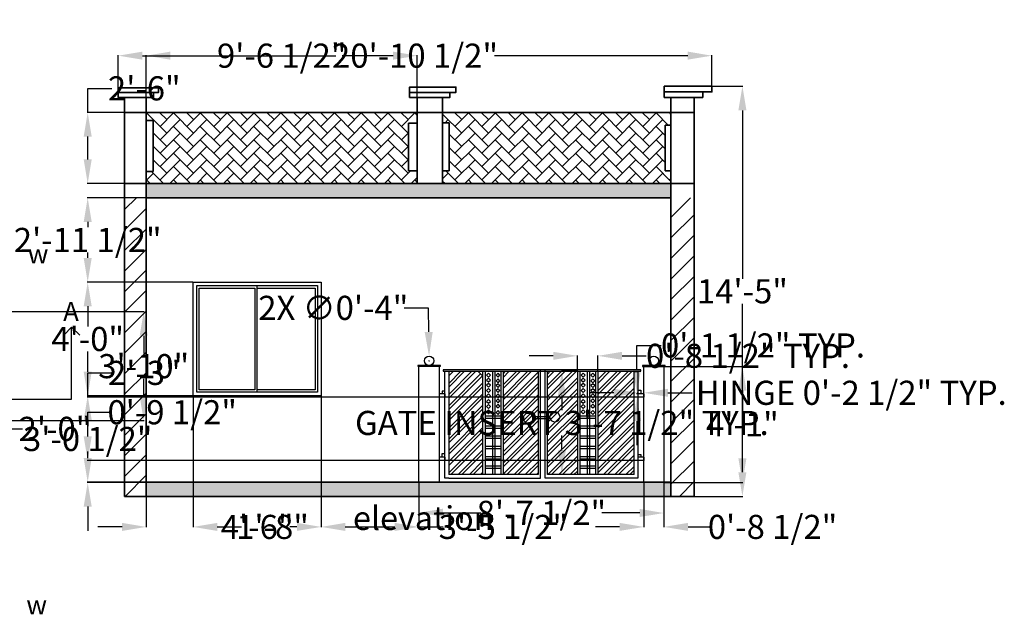
# Model space of a CAD drawing. Units: inches. Extents: x 4451 to 5261, y 886 to 1442.
# Tile 4 of 4: x 4807 to 5223, y 1174 to 1424. Entities that reach past the tile are written whole.
import ezdxf

# ---------------------------------------------------------------- set-up
doc = ezdxf.new("R2010")
doc.units = ezdxf.units.IN
doc.header["$MEASUREMENT"] = 0
for name, color, linetype, lineweight in [('A-ANNO-DIMS', 2, 'Continuous', 18), ('A-ANNO-SYMB', 3, 'Continuous', 25), ('A-ANNO-TEXT', 7, 'Continuous', 25), ('A-ELEV', 7, 'Continuous', 35), ('A-ELEV-GATE', 4, 'Continuous', 25), ('A-GLAZ', 4, 'Continuous', 25)]:
    doc.layers.add(name, color=color, linetype=linetype, lineweight=lineweight)
doc.layers.add('A-ELEV-GATE-PATT', color=30, linetype='Continuous', lineweight=13, true_color=0xf8991e)
doc.layers.add('A-ELEV-PATT', color=240, linetype='Continuous', lineweight=13, true_color=0xed1f24)
doc.styles.get("Standard").update_dxf_attribs({"font": 'arial.ttf'})
doc.dimstyles.get("Standard").update_dxf_attribs({"dimtxt": 10.18, "dimasz": 10.18, "dimexe": 0.18, "dimexo": 0.0625, "dimgap": 0.09, "dimtad": 0, "dimtih": 1, "dimtoh": 1, "dimdec": 0, "dimzin": 0, "dimdsep": 46, "dimlunit": 3, "dimtxsty": 'Standard', "dimcen": 0.09, "dimadec": 0, "dimazin": 0, "dimtfac": 1, "dimtdec": 0, "dimtofl": 0, "dimtmove": 0, "dimatfit": 3, "dimfxl": 1, "dimtolj": 1, "dimtzin": 0, "dimarcsym": 0})
pattern_1 = [(50, (284.271, 536.571), (7.172602, -0.627521), [0.75, -8.25]), (355, (284.271, 536.571), (-1.387513, 7.521921), [0.6, -6.6]), (100.45144, (284.869, 536.519), (5.785088, 6.8944), [0.637402, -7.011421]), (46.1842, (284.271, 538.571), (10.672413, -1.655193), [1.125, -12.375]), (96.63564, (285.16, 538.433), (9.34662, 9.741186), [0.956103, -10.517138]), (351.18416, (284.271, 538.571), (9.34662, 9.741186), [0.9, -9.9]), (21, (285.271, 538.071), (5.9690705, -4.026189), [0.75, -8.25]), (326, (285.271, 538.071), (2.433153, 7.2515), [0.6, -6.6]), (71.45144, (285.7684, 537.7355), (8.402224, 3.225312), [0.637402, -7.011421]), (37.5, (284.271, 536.571), (0.1215986, 3.3289385), [0, -6.52, 0, -6.7, 0, -6.625]), (7.5, (284.271, 536.571), (2.6306954, 3.944117), [0, -3.82, 0, -6.37, 0, -2.525]), (327.5, (282.041, 536.571), (5.3382244, -0.2255487), [0, -2.5, 0, -7.8, 0, -10.35]), (317.5, (281.041, 536.571), (5.8318617, 1.00105), [0, -3.25, 0, -5.18, 0, -7.35])]
pattern_2 = [(45, (284.271, 536.571), (-2.3599689, 2.3599689), []), (45, (285.8443, 536.571), (-2.3599689, 2.3599689), [])]

# ---------------------------------------------------------------- blocks, each defined once
blk = doc.blocks.new('*U9')
for p, q in [((1.5, 1.5), (1.5, 46.5)), ((1.5, 46.5), (27, 46.5)), ((27, 1.5), (27, 46.5)), ((27, 46.5), (52.5, 46.5)), ((52.5, 46.5), (52.5, 1.5)), ((27, 1.5), (1.5, 1.5)), ((52.5, 1.5), (27, 1.5))]:
    blk.add_line(p, q)
blk.add_lwpolyline([(0, 0), (0, 48), (54, 48), (54, 0)], close=True)
for points in [[(26, 45.5), (26, 2.5), (2.5, 2.5), (2.5, 45.5), (26, 45.5)], [(27, 45.5), (51.5, 45.5), (51.5, 2.5), (27, 2.5)]]:
    blk.add_lwpolyline(points)
blk = doc.blocks.new('GATE-ORNAMENTAL-INSERT')
for p, q in [((0, 43.58), (0, 0)), ((1, 43.58), (1, 0)), ((4.1, 43.58), (4.1, 0)), ((5.1, 43.58), (5.1, 0)), ((7.67, 43.58), (7.67, 0)), ((8.67, 43.58), (8.67, 0)), ((1, 24.75), (7.67, 24.75)), ((1, 23.75), (7.67, 23.75)), ((1, 20.57), (7.67, 20.57)), ((1, 19.57), (7.67, 19.57)), ((1, 16.4), (7.67, 16.4)), ((1, 15.4), (7.67, 15.4)), ((1, 12.02), (7.67, 12.02)), ((1, 11.02), (7.67, 11.02)), ((1, 7.67), (7.67, 7.67)), ((1, 6.67), (7.67, 6.67)), ((1, 3.65), (7.67, 3.65)), ((1, 2.65), (7.67, 2.65))]:
    blk.add_line(p, q)
for points in [[(2.44, 41.12), (3.27, 41.95), (2.44, 42.78), (1.61, 41.95)], [(6.48, 41.12), (7.31, 41.95), (6.48, 42.78), (5.65, 41.95)], [(2.44, 39.08), (3.27, 39.9), (2.44, 40.73), (1.61, 39.9)], [(2.44, 36.83), (3.27, 37.66), (2.44, 38.49), (1.61, 37.66)], [(6.48, 38.71), (7.31, 39.54), (6.48, 40.37), (5.65, 39.54)], [(6.48, 36.69), (7.31, 37.52), (6.48, 38.35), (5.65, 37.52)], [(2.44, 34.62), (3.27, 35.45), (2.44, 36.28), (1.61, 35.45)], [(2.44, 32.44), (3.27, 33.26), (2.44, 34.09), (1.61, 33.26)], [(6.48, 34.59), (7.31, 35.42), (6.48, 36.25), (5.65, 35.42)], [(6.48, 32.44), (7.31, 33.27), (6.48, 34.1), (5.65, 33.27)], [(2.44, 30.07), (3.27, 30.9), (2.44, 31.73), (1.61, 30.9)], [(2.44, 27.92), (3.27, 28.74), (2.44, 29.57), (1.61, 28.74)], [(6.48, 30.33), (7.31, 31.16), (6.48, 31.99), (5.65, 31.16)], [(6.48, 28.1), (7.31, 28.93), (6.48, 29.76), (5.65, 28.93)], [(2.44, 25.62), (3.27, 26.45), (2.44, 27.28), (1.61, 26.45)], [(6.48, 25.4), (7.31, 26.23), (6.48, 27.06), (5.65, 26.23)]]:
    blk.add_lwpolyline(points, close=True)
blk = doc.blocks.new('GATE-HINGE-ELEV')
for p, q in [((2.48, 1.41), (0, 1.41)), ((2.48, 1.41), (2.48, 0)), ((2.48, 0), (0, 0))]:
    blk.add_line(p, q)
blk = doc.blocks.new('*D31')
at = {"layer": 'A-ANNO-DIMS', "color": 0, "lineweight": -2, "transparency": 16777216}
for p, q in [((5057.78, 1267), (5047.6, 1267)), ((5067.96, 1266.69), (5067.96, 1267.18)), ((5070.44, 1266.69), (5070.44, 1267.18)), ((5080.62, 1267), (5090.8, 1267))]:
    blk.add_line(p, q, dxfattribs=at)
at = {"layer": 'A-ANNO-DIMS', "color": 0, "transparency": 16777216}
for points in [[(5057.78, 1268.7), (5057.78, 1265.31), (5067.96, 1267)], [(5080.62, 1268.7), (5080.62, 1265.31), (5070.44, 1267)]]:
    blk.add_solid(points, dxfattribs=at)
at = {"layer": 'Defpoints', "color": 0, "transparency": 16777216}
for p in [(5067.96, 1266.63), (5070.44, 1267), (5070.44, 1266.63)]:
    blk.add_point(p, dxfattribs=at)
at = {"layer": 'A-ANNO-DIMS', "color": 0, "transparency": 16777216, "insert": (5158, 1267), "char_height": 10.18, "attachment_point": 5}
blk.add_mtext('\\A1;HINGE 0\'-2 1/2" TYP.', dxfattribs=at)
blk = doc.blocks.new('*D32')
at = {"layer": 'A-ANNO-DIMS', "color": 0, "lineweight": -2, "transparency": 16777216}
for p, q in [((5067.58, 1276.81), (5067.58, 1286.99)), ((5067.58, 1286.99), (5077.76, 1286.99)), ((5067.89, 1266.63), (5067.4, 1266.63)), ((5067.89, 1265.22), (5067.4, 1265.22)), ((5067.58, 1255.04), (5067.58, 1244.86))]:
    blk.add_line(p, q, dxfattribs=at)
at = {"layer": 'A-ANNO-DIMS', "color": 0, "transparency": 16777216}
for points in [[(5065.89, 1276.81), (5069.28, 1276.81), (5067.58, 1266.63)], [(5065.89, 1255.04), (5069.28, 1255.04), (5067.58, 1265.22)]]:
    blk.add_solid(points, dxfattribs=at)
at = {"layer": 'Defpoints', "color": 0, "transparency": 16777216}
for p in [(5067.58, 1266.63), (5067.96, 1266.63), (5067.96, 1265.22)]:
    blk.add_point(p, dxfattribs=at)
at = {"layer": 'A-ANNO-DIMS', "color": 0, "transparency": 16777216, "insert": (5120.74, 1286.99), "char_height": 10.18, "attachment_point": 5}
blk.add_mtext('\\A1;0\'-1 1/2" TYP.', dxfattribs=at)
blk = doc.blocks.new('*D33')
at = {"layer": 'A-ANNO-DIMS', "color": 0, "lineweight": -2, "transparency": 16777216}
for p, q in [((5042.35, 1276.06), (5035.7, 1276.06)), ((5035.88, 1265.88), (5035.88, 1259.63)), ((5035.88, 1242.67), (5035.88, 1248.92)), ((5042.35, 1232.49), (5035.7, 1232.49))]:
    blk.add_line(p, q, dxfattribs=at)
at = {"layer": 'A-ANNO-DIMS', "color": 0, "transparency": 16777216}
for points in [[(5034.18, 1265.88), (5037.57, 1265.88), (5035.88, 1276.06)], [(5034.18, 1242.67), (5037.57, 1242.67), (5035.88, 1232.49)]]:
    blk.add_solid(points, dxfattribs=at)
at = {"layer": 'Defpoints', "color": 0, "transparency": 16777216}
for p in [(5035.88, 1276.06), (5042.41, 1276.06), (5042.41, 1232.49)]:
    blk.add_point(p, dxfattribs=at)
at = {"layer": 'A-ANNO-DIMS', "color": 0, "transparency": 16777216, "insert": (5035.88, 1254.28), "char_height": 10.18, "attachment_point": 5}
blk.add_mtext('\\A1;GATE INSERT 3\'-7 1/2" TYP.', dxfattribs=at)
blk = doc.blocks.new('*D34')
at = {"layer": 'A-ANNO-DIMS', "color": 0, "lineweight": -2, "transparency": 16777216}
for p, q in [((5032.23, 1282.6), (5022.05, 1282.6)), ((5042.41, 1276.13), (5042.41, 1282.78)), ((5051.09, 1276.13), (5051.09, 1282.78)), ((5061.27, 1282.6), (5071.45, 1282.6))]:
    blk.add_line(p, q, dxfattribs=at)
at = {"layer": 'A-ANNO-DIMS', "color": 0, "transparency": 16777216}
for points in [[(5032.23, 1284.3), (5032.23, 1280.9), (5042.41, 1282.6)], [(5061.27, 1284.3), (5061.27, 1280.9), (5051.09, 1282.6)]]:
    blk.add_solid(points, dxfattribs=at)
at = {"layer": 'Defpoints', "color": 0, "transparency": 16777216}
for p in [(5051.09, 1282.6), (5042.41, 1276.06), (5051.09, 1276.06)]:
    blk.add_point(p, dxfattribs=at)
at = {"layer": 'A-ANNO-DIMS', "color": 0, "transparency": 16777216, "insert": (5114.42, 1282.6), "char_height": 10.18, "attachment_point": 5}
blk.add_mtext('\\A1;0\'-8 1/2" TYP.', dxfattribs=at)
blk = doc.blocks.new('*D46')
at = {"layer": 'A-ANNO-DIMS', "color": 0, "lineweight": -2, "transparency": 16777216}
for p, q in [((4798.16, 1301.25), (4859.61, 1301.25)), ((4859.43, 1291.07), (4859.43, 1283.54)), ((4859.43, 1265.43), (4859.43, 1272.96)), ((4798.16, 1255.25), (4859.61, 1255.25))]:
    blk.add_line(p, q, dxfattribs=at)
at = {"layer": 'A-ANNO-DIMS', "color": 0, "transparency": 16777216}
for points in [[(4857.74, 1291.07), (4861.13, 1291.07), (4859.43, 1301.25)], [(4857.74, 1265.43), (4861.13, 1265.43), (4859.43, 1255.25)]]:
    blk.add_solid(points, dxfattribs=at)
at = {"layer": 'Defpoints', "color": 0, "transparency": 16777216}
for p in [(4798.09, 1301.25), (4859.43, 1301.25), (4798.09, 1255.25)]:
    blk.add_point(p, dxfattribs=at)
at = {"layer": 'A-ANNO-DIMS', "color": 0, "transparency": 16777216, "insert": (4859.43, 1278.25), "char_height": 10.18, "attachment_point": 5}
blk.add_mtext('\\A1;3\'-10"', dxfattribs=at)
blk = doc.blocks.new('*D54')
at = {"layer": 'A-ANNO-DIMS', "color": 0, "lineweight": -2, "transparency": 16777216}
for p, q in [((4774.09, 1224.89), (4774.09, 1251.96)), ((4784.27, 1251.78), (4787.91, 1251.78)), ((4798.09, 1224.89), (4798.09, 1251.96)), ((4798.09, 1251.78), (4808.27, 1251.78))]:
    blk.add_line(p, q, dxfattribs=at)
at = {"layer": 'A-ANNO-DIMS', "color": 0, "transparency": 16777216}
for points in [[(4784.27, 1253.48), (4784.27, 1250.08), (4774.09, 1251.78)], [(4787.91, 1253.48), (4787.91, 1250.08), (4798.09, 1251.78)]]:
    blk.add_solid(points, dxfattribs=at)
at = {"layer": 'Defpoints', "color": 0, "transparency": 16777216}
for p in [(4798.09, 1251.78), (4774.09, 1224.83), (4798.09, 1224.83)]:
    blk.add_point(p, dxfattribs=at)
at = {"layer": 'A-ANNO-DIMS', "color": 0, "transparency": 16777216, "insert": (4821.98, 1251.78), "char_height": 10.18, "attachment_point": 5}
blk.add_mtext('\\A1;2\'-0"', dxfattribs=at)
blk = doc.blocks.new('*D57')
at = {"layer": 'A-ANNO-DIMS', "color": 0, "lineweight": -2, "transparency": 16777216}
for p, q in [((4848.69, 1395.83), (4848.69, 1409.46)), ((4858.87, 1409.28), (4940.45, 1409.28)), ((5088.98, 1409.28), (5007.4, 1409.28)), ((5099.16, 1396.45), (5099.16, 1409.46))]:
    blk.add_line(p, q, dxfattribs=at)
at = {"layer": 'A-ANNO-DIMS', "color": 0, "transparency": 16777216}
for points in [[(4858.87, 1410.98), (4858.87, 1407.59), (4848.69, 1409.28)], [(5088.98, 1410.98), (5088.98, 1407.59), (5099.16, 1409.28)]]:
    blk.add_solid(points, dxfattribs=at)
at = {"layer": 'Defpoints', "color": 0, "transparency": 16777216}
for p in [(5099.16, 1409.28), (5099.16, 1396.38), (4848.69, 1395.77)]:
    blk.add_point(p, dxfattribs=at)
at = {"layer": 'A-ANNO-DIMS', "color": 0, "transparency": 16777216, "insert": (4973.92, 1409.28), "char_height": 10.18, "attachment_point": 5}
blk.add_mtext('\\A1;20\'-10 1/2"', dxfattribs=at)
blk = doc.blocks.new('*D58')
at = {"layer": 'A-ANNO-DIMS', "color": 0, "lineweight": -2, "transparency": 16777216}
for p, q in [((5099.22, 1396.38), (5112.24, 1396.38)), ((5112.06, 1386.2), (5112.06, 1315.13)), ((5112.06, 1233.48), (5112.06, 1304.56)), ((5091.77, 1223.3), (5112.24, 1223.3))]:
    blk.add_line(p, q, dxfattribs=at)
at = {"layer": 'A-ANNO-DIMS', "color": 0, "transparency": 16777216}
for points in [[(5110.36, 1386.2), (5113.76, 1386.2), (5112.06, 1396.38)], [(5110.36, 1233.48), (5113.76, 1233.48), (5112.06, 1223.3)]]:
    blk.add_solid(points, dxfattribs=at)
at = {"layer": 'Defpoints', "color": 0, "transparency": 16777216}
for p in [(5099.16, 1396.38), (5112.06, 1396.38), (5091.7, 1223.3)]:
    blk.add_point(p, dxfattribs=at)
at = {"layer": 'A-ANNO-DIMS', "color": 0, "transparency": 16777216, "insert": (5112.06, 1309.84), "char_height": 10.18, "attachment_point": 5}
blk.add_mtext('\\A1;14\'-5"', dxfattribs=at)
blk = doc.blocks.new('*D59')
at = {"layer": 'A-ANNO-DIMS', "color": 0, "lineweight": -2, "transparency": 16777216}
for p, q in [((4860.47, 1385.37), (4860.47, 1409.46)), ((4870.65, 1409.28), (4892.17, 1409.28)), ((4964.65, 1409.28), (4943.13, 1409.28)), ((4974.83, 1380.82), (4974.83, 1409.46))]:
    blk.add_line(p, q, dxfattribs=at)
at = {"layer": 'A-ANNO-DIMS', "color": 0, "transparency": 16777216}
for points in [[(4870.65, 1410.98), (4870.65, 1407.59), (4860.47, 1409.28)], [(4964.65, 1410.98), (4964.65, 1407.59), (4974.83, 1409.28)]]:
    blk.add_solid(points, dxfattribs=at)
at = {"layer": 'Defpoints', "color": 0, "transparency": 16777216}
for p in [(4974.83, 1409.28), (4860.47, 1385.3), (4974.83, 1380.76)]:
    blk.add_point(p, dxfattribs=at)
at = {"layer": 'A-ANNO-DIMS', "color": 0, "transparency": 16777216, "insert": (4917.65, 1409.28), "char_height": 10.18, "attachment_point": 5}
blk.add_mtext('\\A1;9\'-6 1/2"', dxfattribs=at)
blk = doc.blocks.new('*D60')
at = {"layer": 'A-ANNO-DIMS', "color": 0, "lineweight": -2, "transparency": 16777216}
for p, q in [((4835.79, 1385.3), (4835.79, 1395.48)), ((4835.79, 1395.48), (4845.97, 1395.48)), ((4851.29, 1385.3), (4835.61, 1385.3)), ((4835.79, 1365.48), (4835.79, 1375.12)), ((4851.29, 1355.3), (4835.61, 1355.3))]:
    blk.add_line(p, q, dxfattribs=at)
at = {"layer": 'A-ANNO-DIMS', "color": 0, "transparency": 16777216}
for points in [[(4834.09, 1375.12), (4837.48, 1375.12), (4835.79, 1385.3)], [(4834.09, 1365.48), (4837.48, 1365.48), (4835.79, 1355.3)]]:
    blk.add_solid(points, dxfattribs=at)
at = {"layer": 'Defpoints', "color": 0, "transparency": 16777216}
for p in [(4835.79, 1385.3), (4851.36, 1385.3), (4851.36, 1355.3)]:
    blk.add_point(p, dxfattribs=at)
at = {"layer": 'A-ANNO-DIMS', "color": 0, "transparency": 16777216, "insert": (4859.67, 1395.48), "char_height": 10.18, "attachment_point": 5}
blk.add_mtext('\\A1;2\'-6"', dxfattribs=at)
blk = doc.blocks.new('*D61')
at = {"layer": 'A-ANNO-DIMS', "color": 0, "lineweight": -2, "transparency": 16777216}
for p, q in [((4860.41, 1349.3), (4835.61, 1349.3)), ((4835.79, 1339.12), (4835.79, 1336.87)), ((4835.79, 1323.9), (4835.79, 1326.16)), ((4880.22, 1313.72), (4835.61, 1313.72))]:
    blk.add_line(p, q, dxfattribs=at)
at = {"layer": 'A-ANNO-DIMS', "color": 0, "transparency": 16777216}
for points in [[(4834.09, 1339.12), (4837.48, 1339.12), (4835.79, 1349.3)], [(4834.09, 1323.9), (4837.48, 1323.9), (4835.79, 1313.72)]]:
    blk.add_solid(points, dxfattribs=at)
at = {"layer": 'Defpoints', "color": 0, "transparency": 16777216}
for p in [(4835.79, 1349.3), (4860.47, 1349.3), (4880.28, 1313.72)]:
    blk.add_point(p, dxfattribs=at)
at = {"layer": 'A-ANNO-DIMS', "color": 0, "transparency": 16777216, "insert": (4835.79, 1331.51), "char_height": 10.18, "attachment_point": 5}
blk.add_mtext('\\A1;2\'-11 1/2"', dxfattribs=at)
blk = doc.blocks.new('*D62')
at = {"layer": 'A-ANNO-DIMS', "color": 0, "lineweight": -2, "transparency": 16777216}
for p, q in [((4880.22, 1313.72), (4835.61, 1313.72)), ((4835.79, 1303.54), (4835.79, 1295.01)), ((4835.79, 1275.9), (4835.79, 1284.44)), ((4880.22, 1265.72), (4835.61, 1265.72))]:
    blk.add_line(p, q, dxfattribs=at)
at = {"layer": 'A-ANNO-DIMS', "color": 0, "transparency": 16777216}
for points in [[(4834.09, 1303.54), (4837.48, 1303.54), (4835.79, 1313.72)], [(4834.09, 1275.9), (4837.48, 1275.9), (4835.79, 1265.72)]]:
    blk.add_solid(points, dxfattribs=at)
at = {"layer": 'Defpoints', "color": 0, "transparency": 16777216}
for p in [(4835.79, 1313.72), (4880.28, 1313.72), (4880.28, 1265.72)]:
    blk.add_point(p, dxfattribs=at)
at = {"layer": 'A-ANNO-DIMS', "color": 0, "transparency": 16777216, "insert": (4835.79, 1289.72), "char_height": 10.18, "attachment_point": 5}
blk.add_mtext('\\A1;4\'-0"', dxfattribs=at)
blk = doc.blocks.new('*D63')
at = {"layer": 'A-ANNO-DIMS', "color": 0, "lineweight": -2, "transparency": 16777216}
for p, q in [((4880.22, 1265.72), (4835.61, 1265.72)), ((4835.79, 1255.54), (4835.79, 1252.87)), ((4835.79, 1239.48), (4835.79, 1242.16)), ((4860.41, 1229.3), (4835.61, 1229.3))]:
    blk.add_line(p, q, dxfattribs=at)
at = {"layer": 'A-ANNO-DIMS', "color": 0, "transparency": 16777216}
for points in [[(4834.09, 1255.54), (4837.48, 1255.54), (4835.79, 1265.72)], [(4834.09, 1239.48), (4837.48, 1239.48), (4835.79, 1229.3)]]:
    blk.add_solid(points, dxfattribs=at)
at = {"layer": 'Defpoints', "color": 0, "transparency": 16777216}
for p in [(4835.79, 1265.72), (4880.28, 1265.72), (4860.47, 1229.3)]:
    blk.add_point(p, dxfattribs=at)
at = {"layer": 'A-ANNO-DIMS', "color": 0, "transparency": 16777216, "insert": (4835.79, 1247.51), "char_height": 10.18, "attachment_point": 5}
blk.add_mtext('\\A1;3\'-0 1/2"', dxfattribs=at)
blk = doc.blocks.new('*D64')
at = {"layer": 'A-ANNO-DIMS', "color": 0, "lineweight": -2, "transparency": 16777216}
for p, q in [((4880.28, 1265.66), (4880.28, 1210.22)), ((4860.47, 1229.24), (4860.47, 1210.22)), ((4850.29, 1210.4), (4840.11, 1210.4)), ((4890.46, 1210.4), (4900.64, 1210.4))]:
    blk.add_line(p, q, dxfattribs=at)
at = {"layer": 'A-ANNO-DIMS', "color": 0, "transparency": 16777216}
for points in [[(4850.29, 1212.1), (4850.29, 1208.71), (4860.47, 1210.4)], [(4890.46, 1212.1), (4890.46, 1208.71), (4880.28, 1210.4)]]:
    blk.add_solid(points, dxfattribs=at)
at = {"layer": 'Defpoints', "color": 0, "transparency": 16777216}
for p in [(4880.28, 1265.72), (4860.47, 1229.3), (4880.28, 1210.4)]:
    blk.add_point(p, dxfattribs=at)
at = {"layer": 'A-ANNO-DIMS', "color": 0, "transparency": 16777216, "insert": (4913.79, 1210.4), "char_height": 10.18, "attachment_point": 5}
blk.add_mtext('\\A1;1\'-8"', dxfattribs=at)
blk = doc.blocks.new('*D65')
at = {"layer": 'A-ANNO-DIMS', "color": 0, "lineweight": -2, "transparency": 16777216}
for p, q in [((4880.28, 1265.66), (4880.28, 1210.22)), ((4934.28, 1265.66), (4934.28, 1210.22)), ((4890.46, 1210.4), (4893.46, 1210.4)), ((4924.1, 1210.4), (4921.11, 1210.4))]:
    blk.add_line(p, q, dxfattribs=at)
at = {"layer": 'A-ANNO-DIMS', "color": 0, "transparency": 16777216}
for points in [[(4890.46, 1212.1), (4890.46, 1208.71), (4880.28, 1210.4)], [(4924.1, 1212.1), (4924.1, 1208.71), (4934.28, 1210.4)]]:
    blk.add_solid(points, dxfattribs=at)
at = {"layer": 'Defpoints', "color": 0, "transparency": 16777216}
for p in [(4880.28, 1265.72), (4934.28, 1265.72), (4934.28, 1210.4)]:
    blk.add_point(p, dxfattribs=at)
at = {"layer": 'A-ANNO-DIMS', "color": 0, "transparency": 16777216, "insert": (4907.28, 1210.4), "char_height": 10.18, "attachment_point": 5}
blk.add_mtext('\\A1;4\'-6"', dxfattribs=at)
blk = doc.blocks.new('*D66')
at = {"layer": 'A-ANNO-DIMS', "color": 0, "lineweight": -2, "transparency": 16777216}
for p, q in [((4934.28, 1265.66), (4934.28, 1210.22)), ((4975.57, 1229.24), (4975.57, 1210.22)), ((4944.46, 1210.4), (4965.39, 1210.4)), ((4975.57, 1210.4), (4985.75, 1210.4))]:
    blk.add_line(p, q, dxfattribs=at)
at = {"layer": 'A-ANNO-DIMS', "color": 0, "transparency": 16777216}
for points in [[(4944.46, 1212.1), (4944.46, 1208.71), (4934.28, 1210.4)], [(4965.39, 1212.1), (4965.39, 1208.71), (4975.57, 1210.4)]]:
    blk.add_solid(points, dxfattribs=at)
at = {"layer": 'Defpoints', "color": 0, "transparency": 16777216}
for p in [(4934.28, 1265.72), (4975.57, 1229.3), (4975.57, 1210.4)]:
    blk.add_point(p, dxfattribs=at)
at = {"layer": 'A-ANNO-DIMS', "color": 0, "transparency": 16777216, "insert": (5011.23, 1210.4), "char_height": 10.18, "attachment_point": 5}
blk.add_mtext('\\A1;3\'-5 1/2"', dxfattribs=at)
blk = doc.blocks.new('*D67')
at = {"layer": 'A-ANNO-DIMS', "color": 0, "lineweight": -2, "transparency": 16777216}
for p, q in [((4975.57, 1229.24), (4975.56, 1216.22)), ((5078.94, 1229.1), (5078.92, 1216.08)), ((4985.74, 1216.39), (5001.75, 1216.37)), ((5068.74, 1216.27), (5052.73, 1216.3))]:
    blk.add_line(p, q, dxfattribs=at)
at = {"layer": 'A-ANNO-DIMS', "color": 0, "transparency": 16777216}
for points in [[(4985.74, 1218.09), (4985.73, 1214.69), (4975.56, 1216.4)], [(5068.74, 1217.97), (5068.74, 1214.58), (5078.92, 1216.26)]]:
    blk.add_solid(points, dxfattribs=at)
at = {"layer": 'Defpoints', "color": 0, "transparency": 16777216}
for p in [(4975.57, 1229.3), (5078.94, 1229.16), (4975.56, 1216.4)]:
    blk.add_point(p, dxfattribs=at)
at = {"layer": 'A-ANNO-DIMS', "color": 0, "transparency": 16777216, "insert": (5027.24, 1216.33), "char_height": 10.18, "attachment_point": 5}
blk.add_mtext('\\A1;8\'-7 1/2"', dxfattribs=at)
blk = doc.blocks.new('*D68')
at = {"layer": 'A-ANNO-DIMS', "color": 0, "lineweight": -2, "transparency": 16777216}
for p, q in [((5079, 1278.14), (5112.24, 1278.14)), ((5112.06, 1267.96), (5112.06, 1258.85)), ((5112.06, 1239.34), (5112.06, 1248.45)), ((5079, 1229.16), (5112.24, 1229.16))]:
    blk.add_line(p, q, dxfattribs=at)
at = {"layer": 'A-ANNO-DIMS', "color": 0, "transparency": 16777216}
for points in [[(5110.36, 1267.96), (5113.76, 1267.96), (5112.06, 1278.14)], [(5110.36, 1239.34), (5113.76, 1239.34), (5112.06, 1229.16)]]:
    blk.add_solid(points, dxfattribs=at)
at = {"layer": 'Defpoints', "color": 0, "transparency": 16777216}
for p in [(5078.94, 1278.14), (5112.06, 1278.14), (5078.94, 1229.16)]:
    blk.add_point(p, dxfattribs=at)
at = {"layer": 'A-ANNO-DIMS', "color": 0, "transparency": 16777216, "insert": (5112.06, 1253.65), "char_height": 10.18, "attachment_point": 5}
blk.add_mtext('\\A1;4\'-1"', dxfattribs=at)
blk = doc.blocks.new('*D69')
at = {"layer": 'A-ANNO-DIMS', "color": 0, "lineweight": -2, "transparency": 16777216}
for p, q in [((4835.79, 1248.61), (4835.79, 1258.79)), ((4835.79, 1258.79), (4845.97, 1258.79)), ((5070.38, 1238.43), (4835.61, 1238.43)), ((5070.38, 1229.16), (4835.61, 1229.16)), ((4835.79, 1218.98), (4835.79, 1208.8))]:
    blk.add_line(p, q, dxfattribs=at)
at = {"layer": 'A-ANNO-DIMS', "color": 0, "transparency": 16777216}
for points in [[(4834.09, 1248.61), (4837.48, 1248.61), (4835.79, 1238.43)], [(4834.09, 1218.98), (4837.48, 1218.98), (4835.79, 1229.16)]]:
    blk.add_solid(points, dxfattribs=at)
at = {"layer": 'Defpoints', "color": 0, "transparency": 16777216}
for p in [(4835.79, 1238.43), (5070.44, 1238.43), (5070.44, 1229.16)]:
    blk.add_point(p, dxfattribs=at)
at = {"layer": 'A-ANNO-DIMS', "color": 0, "transparency": 16777216, "insert": (4871.45, 1258.79), "char_height": 10.18, "attachment_point": 5}
blk.add_mtext('\\A1;0\'-9 1/2"', dxfattribs=at)
blk = doc.blocks.new('*D70')
at = {"layer": 'A-ANNO-DIMS', "color": 0, "lineweight": -2, "transparency": 16777216}
for p, q in [((4835.79, 1265.22), (4835.79, 1275.4)), ((4835.79, 1275.4), (4845.97, 1275.4)), ((5070.38, 1265.22), (4835.61, 1265.22)), ((4835.79, 1248.61), (4835.79, 1255.04)), ((5070.38, 1238.43), (4835.61, 1238.43))]:
    blk.add_line(p, q, dxfattribs=at)
at = {"layer": 'A-ANNO-DIMS', "color": 0, "transparency": 16777216}
for points in [[(4834.09, 1255.04), (4837.48, 1255.04), (4835.79, 1265.22)], [(4834.09, 1248.61), (4837.48, 1248.61), (4835.79, 1238.43)]]:
    blk.add_solid(points, dxfattribs=at)
at = {"layer": 'Defpoints', "color": 0, "transparency": 16777216}
for p in [(4835.79, 1265.22), (5070.44, 1265.22), (5070.44, 1238.43)]:
    blk.add_point(p, dxfattribs=at)
at = {"layer": 'A-ANNO-DIMS', "color": 0, "transparency": 16777216, "insert": (4859.67, 1275.4), "char_height": 10.18, "attachment_point": 5}
blk.add_mtext('\\A1;2\'-3"', dxfattribs=at)
blk = doc.blocks.new('*D71')
at = {"layer": 'A-ANNO-DIMS', "color": 0, "lineweight": -2, "transparency": 16777216}
for p, q in [((5070.44, 1229.1), (5070.44, 1210.22)), ((5078.94, 1229.1), (5078.94, 1210.22)), ((5060.26, 1210.4), (5050.08, 1210.4)), ((5089.12, 1210.4), (5099.3, 1210.4))]:
    blk.add_line(p, q, dxfattribs=at)
at = {"layer": 'A-ANNO-DIMS', "color": 0, "transparency": 16777216}
for points in [[(5060.26, 1212.1), (5060.26, 1208.71), (5070.44, 1210.4)], [(5089.12, 1212.1), (5089.12, 1208.71), (5078.94, 1210.4)]]:
    blk.add_solid(points, dxfattribs=at)
at = {"layer": 'Defpoints', "color": 0, "transparency": 16777216}
for p in [(5070.44, 1229.16), (5078.94, 1229.16), (5078.94, 1210.4)]:
    blk.add_point(p, dxfattribs=at)
at = {"layer": 'A-ANNO-DIMS', "color": 0, "transparency": 16777216, "insert": (5124.78, 1210.4), "char_height": 10.18, "attachment_point": 5}
blk.add_mtext('\\A1;0\'-8 1/2"', dxfattribs=at)
blk = doc.blocks.new('*D84')
at = {"layer": 'A-ANNO-DIMS', "color": 0, "lineweight": -2, "transparency": 16777216}
for p, q in [((4969.33, 1302.85), (4979.51, 1302.85)), ((4979.51, 1302.85), (4979.67, 1292.67)), ((4979.78, 1280.51), (4979.96, 1280.51)), ((4979.87, 1280.42), (4979.87, 1280.6))]:
    blk.add_line(p, q, dxfattribs=at)
at = {"layer": 'A-ANNO-DIMS', "color": 0, "transparency": 16777216}
blk.add_solid([(4981.37, 1292.7), (4977.98, 1292.64), (4979.84, 1282.49)], dxfattribs=at)
at = {"layer": 'Defpoints', "color": 0, "transparency": 16777216}
for p in [(4979.84, 1282.49), (4979.91, 1278.53)]:
    blk.add_point(p, dxfattribs=at)
at = {"layer": 'A-ANNO-DIMS', "color": 0, "transparency": 16777216, "insert": (4939.42, 1302.85), "char_height": 10.18, "attachment_point": 5}
blk.add_mtext('\\A1;2X ∅0\'-4"', dxfattribs=at)

msp = doc.modelspace()

# ---------------------------------------------------------------- hatches: boundary and pattern name
at = {"layer": 'A-ELEV-GATE-PATT'}
h = msp.add_hatch(dxfattribs=at)
h.set_pattern_fill('ANSI32', color=256, scale=8.9)
h.set_pattern_definition(pattern_2)
h.paths.add_polyline_path([(4988.16, 1232.49), (5002.45, 1232.49), (5002.45, 1274.16), (5000.43, 1276.06), (4988.16, 1276.06)])
h.paths.add_polyline_path([(5025.85, 1276.06), (5011.12, 1276.06), (5011.12, 1232.49), (5025.85, 1232.49)])
h.paths.add_polyline_path([(5051.09, 1232.49), (5066.35, 1232.49), (5066.35, 1276.06), (5051.09, 1276.06)])
h.paths.add_polyline_path([(5029.85, 1232.49), (5042.41, 1232.49), (5042.41, 1276.06), (5029.85, 1276.06)])
h = msp.add_hatch(dxfattribs=at)
h.set_pattern_fill('ANSI32', color=256, scale=8.9)
h.set_pattern_definition(pattern_2)
h.paths.add_polyline_path([(5025.85, 1276.06), (5011.12, 1276.06), (5011.12, 1232.49), (5025.85, 1232.49)])
at = {"layer": 'A-ELEV-PATT'}
h = msp.add_hatch(dxfattribs=at)
h.set_pattern_fill('AR-HBONE', color=256)
h.set_pattern_definition([(45, (284.271, 536.571), (0, 5.6568542), [12, -4]), (135, (287.0994, 539.3994), (4e-16, 5.6568542), [12, -4])])
h.paths.add_polyline_path([(4860.47, 1385.3), (4860.47, 1381.96), (4863.44, 1381.96), (4863.44, 1360.4), (4860.47, 1360.4), (4860.47, 1355.3), (4974.83, 1355.3), (4974.83, 1360.65), (4971.11, 1360.65), (4971.11, 1380.76), (4974.83, 1380.76), (4974.83, 1385.3)])
h.paths.add_polyline_path([(5081.92, 1355.3), (5081.92, 1360.65), (5079.5, 1360.65), (5079.5, 1379.97), (5081.92, 1379.97), (5081.92, 1385.3), (4985.57, 1385.3), (4985.57, 1380.92), (4988.38, 1380.92), (4988.38, 1360.65), (4985.57, 1360.65), (4985.57, 1355.3)])
h = msp.add_hatch(dxfattribs=at)
h.set_pattern_fill('AR-CONC', color=256)
h.set_pattern_definition(pattern_1)
h.paths.add_polyline_path([(4979.22, 1355.3), (4860.47, 1355.3), (4860.47, 1349.3), (4979.22, 1349.3)])
h.paths.add_polyline_path([(5081.92, 1355.3), (4979.22, 1355.3), (4979.22, 1349.3), (5081.92, 1349.3)])
h = msp.add_hatch(dxfattribs=at)
h.set_pattern_fill('ANSI31', color=256, scale=49)
h.set_pattern_definition([(45, (284.271, 536.571), (-4.331029, 4.331029), [])])
h.paths.add_polyline_path([(4860.47, 1349.3), (4851.36, 1349.3), (4851.36, 1223.3), (4860.47, 1223.3)])
h.paths.add_polyline_path([(5091.7, 1349.3), (5081.92, 1349.3), (5081.92, 1223.3), (5091.7, 1223.3)])
h = msp.add_hatch(dxfattribs=at)
h.set_pattern_fill('AR-CONC', color=256)
h.set_pattern_definition(pattern_1)
h.paths.add_polyline_path([(5081.92, 1223.3), (5081.92, 1229.3), (4860.47, 1229.3), (4860.47, 1223.3)])

# ---------------------------------------------------------------- linework, layer by layer
at = {"layer": 'A-ANNO-SYMB'}
for p, q in [((4828.9, 1294.64), (4825.87, 1291.41)), ((4828.9, 1264.36), (4828.9, 1294.64)), ((4828.9, 1294.64), (4832.48, 1291.28)), ((4671.09, 1264.36), (4828.9, 1264.36))]:
    msp.add_line(p, q, dxfattribs=at)
at = {"layer": 'A-ELEV'}
for p, q in [((4860.47, 1391.69), (4851.36, 1391.69)), ((4851.36, 1385.3), (4851.36, 1391.69)), ((4860.47, 1385.3), (4860.47, 1391.69)), ((5081.92, 1391.69), (5091.7, 1391.69)), ((5081.92, 1385.3), (5081.92, 1391.69)), ((5091.7, 1391.69), (5091.7, 1385.3)), ((4851.36, 1385.3), (4851.36, 1223.3)), ((4851.36, 1385.3), (5091.7, 1385.3)), ((4860.47, 1385.3), (4860.47, 1223.3)), ((5081.92, 1385.3), (5081.92, 1223.3)), ((5091.7, 1385.3), (5091.7, 1223.3)), ((4860.47, 1381.96), (4863.44, 1381.96)), ((4863.44, 1381.96), (4863.44, 1360.4)), ((4974.83, 1380.76), (4971.11, 1380.76)), ((4971.11, 1380.76), (4971.11, 1360.65)), ((4985.57, 1380.92), (4988.38, 1380.92)), ((4988.38, 1380.92), (4988.38, 1360.65)), ((5081.92, 1379.97), (5079.5, 1379.97)), ((5079.5, 1379.97), (5079.5, 1360.65)), ((4863.44, 1360.4), (4860.47, 1360.4)), ((4971.11, 1360.65), (4974.83, 1360.65)), ((4988.38, 1360.65), (4985.57, 1360.65)), ((5079.5, 1360.65), (5081.92, 1360.65)), ((4851.36, 1355.3), (5091.7, 1355.3)), ((4860.47, 1349.3), (5081.92, 1349.3)), ((4860.47, 1229.3), (5081.92, 1229.3)), ((4851.36, 1223.3), (5091.7, 1223.3))]:
    msp.add_line(p, q, dxfattribs=at)
for points in [[(5079.07, 1393.98), (5079.07, 1393.98), (5099.16, 1393.98), (5099.16, 1393.98), (5099.16, 1396.38), (5099.16, 1396.38), (5079.07, 1396.38), (5079.07, 1396.38)], [(4848.69, 1393.72), (4848.69, 1393.72), (4865.66, 1393.72), (4865.66, 1393.72), (4865.66, 1395.77), (4865.66, 1395.77), (4848.69, 1395.77), (4848.69, 1395.77)], [(4848.69, 1391.64), (4848.69, 1391.64), (4863.58, 1391.64), (4863.58, 1391.64), (4863.58, 1393.72), (4863.58, 1393.72), (4848.69, 1393.72), (4848.69, 1393.72)], [(4971.6, 1393.78), (4971.6, 1393.78), (4991.18, 1393.78), (4991.18, 1393.78), (4991.18, 1395.99), (4991.18, 1395.99), (4971.6, 1395.99), (4971.6, 1395.99)], [(4971.6, 1391.69), (4971.6, 1391.69), (4988.65, 1391.69), (4988.65, 1391.69), (4988.65, 1393.78), (4988.65, 1393.78), (4971.6, 1393.78), (4971.6, 1393.78)], [(5079.07, 1391.69), (5079.07, 1391.69), (5095.3, 1391.69), (5095.3, 1391.69), (5095.3, 1393.98), (5095.3, 1393.98), (5079.07, 1393.98), (5079.07, 1393.98)], [(4974.83, 1355.3), (4974.83, 1355.3), (4985.57, 1355.3), (4985.57, 1355.3), (4985.57, 1391.69), (4985.57, 1391.69), (4974.83, 1391.69), (4974.83, 1391.69)]]:
    msp.add_lwpolyline(points, close=True, dxfattribs=at)
at = {"layer": 'A-ELEV-GATE'}
for p, q in [((5000.43, 1276.06), (5002.45, 1274.16)), ((5028.85, 1232.49), (5028.85, 1276.64)), ((5029.85, 1232.49), (5029.85, 1276.06)), ((4986.56, 1267.71), (4985.35, 1267.71)), ((4985.35, 1267.71), (4985.35, 1266.63)), ((5067.96, 1268.08), (5069.14, 1268.08)), ((5069.14, 1268.08), (5069.14, 1266.63)), ((4984.07, 1266.55), (4984.07, 1266.55)), ((4986.56, 1241.22), (4985.18, 1241.22)), ((4985.18, 1241.22), (4985.18, 1239.84)), ((5067.96, 1240.9), (5069.17, 1240.9)), ((5069.17, 1240.9), (5069.17, 1239.84)), ((5028.85, 1230.93), (5028.85, 1232.49)), ((5066.35, 1230.93), (5028.85, 1230.93)), ((5066.35, 1232.49), (5029.85, 1232.49))]:
    msp.add_line(p, q, dxfattribs=at)
for points in [[(4975.09, 1278.29), (4975.09, 1278.29), (4984.66, 1278.29), (4984.66, 1278.29), (4984.66, 1278.53), (4984.66, 1278.53), (4975.09, 1278.53), (4975.09, 1278.53)], [(4984.07, 1229.3), (4984.07, 1229.3), (4975.57, 1229.3), (4975.57, 1229.3), (4975.57, 1278.29), (4975.57, 1278.29), (4984.07, 1278.29), (4984.07, 1278.29)], [(4985.8, 1276.06), (4985.8, 1276.06), (5069.18, 1276.06), (5069.18, 1276.06), (5069.18, 1276.64), (5069.18, 1276.64), (4985.8, 1276.64), (4985.8, 1276.64)], [(5069.92, 1278.14), (5069.92, 1278.14), (5079.42, 1278.14), (5079.42, 1278.14), (5079.42, 1278.56), (5079.42, 1278.56), (5069.92, 1278.56), (5069.92, 1278.56)], [(5078.94, 1229.16), (5078.94, 1229.16), (5070.44, 1229.16), (5070.44, 1229.16), (5070.44, 1278.14), (5070.44, 1278.14), (5078.94, 1278.14), (5078.94, 1278.14)], [(5031.32, 1258.44), (5030.67, 1256.86), (5031.32, 1255.29), (5032.9, 1254.64), (5034.47, 1255.29), (5035.12, 1256.86), (5034.47, 1258.44), (5032.9, 1259.09)], [(5020.76, 1254.32), (5022.39, 1254.3), (5023.56, 1255.43), (5023.59, 1257.06), (5022.45, 1258.23), (5020.82, 1258.26), (5019.65, 1257.12), (5019.63, 1255.49)], [(5023.59, 1257.06), (5023.59, 1257.06), (5030.63, 1257.06), (5030.63, 1257.06), (5030.63, 1256.08), (5030.63, 1256.08), (5023.59, 1256.08), (5023.59, 1256.08)]]:
    msp.add_lwpolyline(points, close=True, dxfattribs=at)
for points in [[(4988.16, 1230.95), (4988.16, 1230.95), (4986.56, 1230.95), (4986.56, 1230.95), (4986.56, 1276.06), (4986.56, 1276.06), (4988.16, 1276.06), (4988.16, 1276.06), (4988.16, 1232.49)], [(4988.16, 1230.95), (4988.16, 1230.95), (5026.85, 1230.95), (5026.85, 1276.64)], [(5025.85, 1276.06), (5025.85, 1232.49), (4988.16, 1232.49), (4988.16, 1232.49)], [(5066.35, 1232.49), (5066.35, 1276.04), (5066.35, 1276.04), (5067.96, 1276.04), (5067.96, 1276.04), (5067.96, 1230.93), (5067.96, 1230.93), (5066.35, 1230.93), (5066.35, 1230.93), (5066.35, 1230.95)]]:
    msp.add_lwpolyline(points, dxfattribs=at)
for centre in [(4979.87, 1280.51), (5074.67, 1280.54)]:
    msp.add_circle(centre, 1.98, dxfattribs=at)

# ---------------------------------------------------------------- block references
for name, p in [('GATE-ORNAMENTAL-INSERT', (5002.45, 1232.49)), ('GATE-ORNAMENTAL-INSERT', (5042.41, 1232.49)), ('GATE-HINGE-ELEV', (4984.07, 1265.22)), ('GATE-HINGE-ELEV', (5067.96, 1265.22)), ('GATE-HINGE-ELEV', (4984.07, 1238.43)), ('GATE-HINGE-ELEV', (5067.96, 1238.43))]:
    msp.add_blockref(name, p, dxfattribs=at)
at = {"layer": 'A-GLAZ'}
msp.add_blockref('*U9', (4880.28, 1265.72), dxfattribs=at)

# ---------------------------------------------------------------- texts
at = {"layer": 'A-ANNO-SYMB', "insert": (4825.42, 1305.3), "char_height": 8, "attachment_point": 1}
msp.add_mtext_dynamic_manual_height_columns('A', width=18.4117, gutter_width=1, heights=[0], dxfattribs=at)
at = {"layer": 'A-ANNO-TEXT', "attachment_point": 1}
for s, width, insert, char_height in [('w', 18.4117, (4810.47, 1329.68), 8), ('elevation', 120.4981, (4947.73, 1219.1), 10), ('w', 18.4117, (4809.88, 1181.51), 8)]:
    msp.add_mtext_dynamic_manual_height_columns(s, width=width, gutter_width=1, heights=[0], dxfattribs=dict(at, insert=insert, char_height=char_height))

# ---------------------------------------------------------------- dimensions: what is measured, and where the dimension line sits
at = {"layer": 'A-ANNO-DIMS'}
for base, p1, p2, picture, middle in [((5099.16, 1409.28), (4848.69, 1395.77), (5099.16, 1396.38), '*D57', (4973.92, 1409.28)), ((4974.83, 1409.28), (4860.47, 1385.3), (4974.83, 1380.76), '*D59', (4917.65, 1409.28)), ((4880.28, 1210.4), (4860.47, 1229.3), (4880.28, 1265.72), '*D64', (4913.79, 1210.4)), ((4934.28, 1210.4), (4880.28, 1265.72), (4934.28, 1265.72), '*D65', (4907.28, 1210.4)), ((4975.57, 1210.4), (4934.28, 1265.72), (4975.57, 1229.3), '*D66', (5011.23, 1210.4)), ((4798.09, 1251.78), (4774.09, 1224.83), (4798.09, 1224.83), '*D54', (4821.98, 1251.78)), ((5078.94, 1210.4), (5070.44, 1229.16), (5078.94, 1229.16), '*D71', (5124.78, 1210.4))]:
    dim = msp.add_linear_dim(base=base, p1=p1, p2=p2, dimstyle='Standard', override={"dimdec": 1, "dimlfac": 1, "dimrnd": 0, "dimzin": 1, "dimdsep": 46, "dimlunit": 4, "dimfrac": 2}, dxfattribs=at)
    dim.commit()
    dim.dimension.update_dxf_attribs({"geometry": picture, "text_midpoint": middle})
for base, p1, p2, angle, picture, middle in [((4835.79, 1385.3), (4851.36, 1355.3), (4851.36, 1385.3), 90, '*D60', (4859.67, 1395.48)), ((5112.06, 1396.38), (5091.7, 1223.3), (5099.16, 1396.38), 90, '*D58', (5112.06, 1309.84)), ((4835.79, 1349.3), (4880.28, 1313.72), (4860.47, 1349.3), 90, '*D61', (4835.79, 1331.51)), ((4835.79, 1313.72), (4880.28, 1265.72), (4880.28, 1313.72), 90, '*D62', (4835.79, 1289.72)), ((4859.43, 1301.25), (4798.09, 1255.25), (4798.09, 1301.25), 90, '*D46', (4859.43, 1278.25)), ((4835.79, 1265.22), (5070.44, 1238.43), (5070.44, 1265.22), 90, '*D70', (4859.67, 1275.4)), ((5112.06, 1278.14), (5078.94, 1229.16), (5078.94, 1278.14), 90, '*D68', (5112.06, 1253.65)), ((4835.79, 1238.43), (5070.44, 1229.16), (5070.44, 1238.43), 90, '*D69', (4871.45, 1258.79)), ((4835.79, 1265.72), (4860.47, 1229.3), (4880.28, 1265.72), 90, '*D63', (4835.79, 1247.51)), ((4975.56, 1216.4), (5078.94, 1229.16), (4975.57, 1229.3), 179.9193, '*D67', (5027.24, 1216.33))]:
    dim = msp.add_linear_dim(base=base, p1=p1, p2=p2, angle=angle, dimstyle='Standard', override={"dimdec": 1, "dimlfac": 1, "dimrnd": 0, "dimzin": 1, "dimdsep": 46, "dimlunit": 4, "dimfrac": 2}, dxfattribs=at)
    dim.commit()
    dim.dimension.update_dxf_attribs({"geometry": picture, "text_midpoint": middle})
dim = msp.add_diameter_dim_2p(p1=(4979.91, 1278.53), p2=(4979.84, 1282.49), text='2X <>', dimstyle='Standard', override={"dimdec": 1, "dimlfac": 1, "dimrnd": 0, "dimzin": 1, "dimdsep": 46, "dimlunit": 4, "dimfrac": 2}, dxfattribs=at)
dim.commit()
dim.dimension.update_dxf_attribs({"geometry": '*D84', "text_midpoint": (4939.42, 1302.85)})
for base, p1, p2, text, picture, middle in [((5067.58, 1266.63), (5067.96, 1265.22), (5067.96, 1266.63), '<> TYP.', '*D32', (5120.74, 1286.99)), ((5035.88, 1276.06), (5042.41, 1232.49), (5042.41, 1276.06), 'GATE INSERT <> TYP.', '*D33', (5035.88, 1254.28))]:
    dim = msp.add_linear_dim(base=base, p1=p1, p2=p2, angle=90, text=text, dimstyle='Standard', override={"dimdec": 1, "dimlfac": 1, "dimrnd": 0, "dimzin": 1, "dimdsep": 46, "dimlunit": 4, "dimfrac": 2}, dxfattribs=at)
    dim.commit()
    dim.dimension.update_dxf_attribs({"geometry": picture, "text_midpoint": middle})
for base, p1, p2, text, picture, middle in [((5051.09, 1282.6), (5042.41, 1276.06), (5051.09, 1276.06), '<> TYP.', '*D34', (5114.42, 1282.6)), ((5070.44, 1267), (5067.96, 1266.63), (5070.44, 1266.63), 'HINGE <> TYP.', '*D31', (5158, 1267))]:
    dim = msp.add_linear_dim(base=base, p1=p1, p2=p2, text=text, dimstyle='Standard', override={"dimdec": 1, "dimlfac": 1, "dimrnd": 0, "dimzin": 1, "dimdsep": 46, "dimlunit": 4, "dimfrac": 2}, dxfattribs=at)
    dim.commit()
    dim.dimension.update_dxf_attribs({"geometry": picture, "text_midpoint": middle})

doc.saveas('drawing.dxf')
